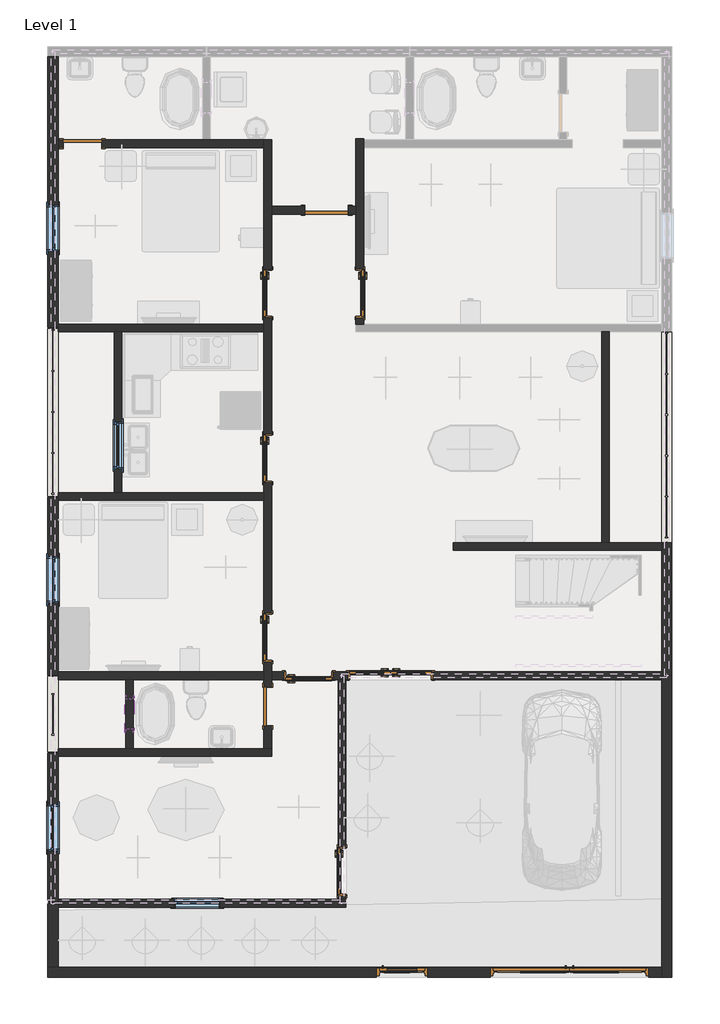
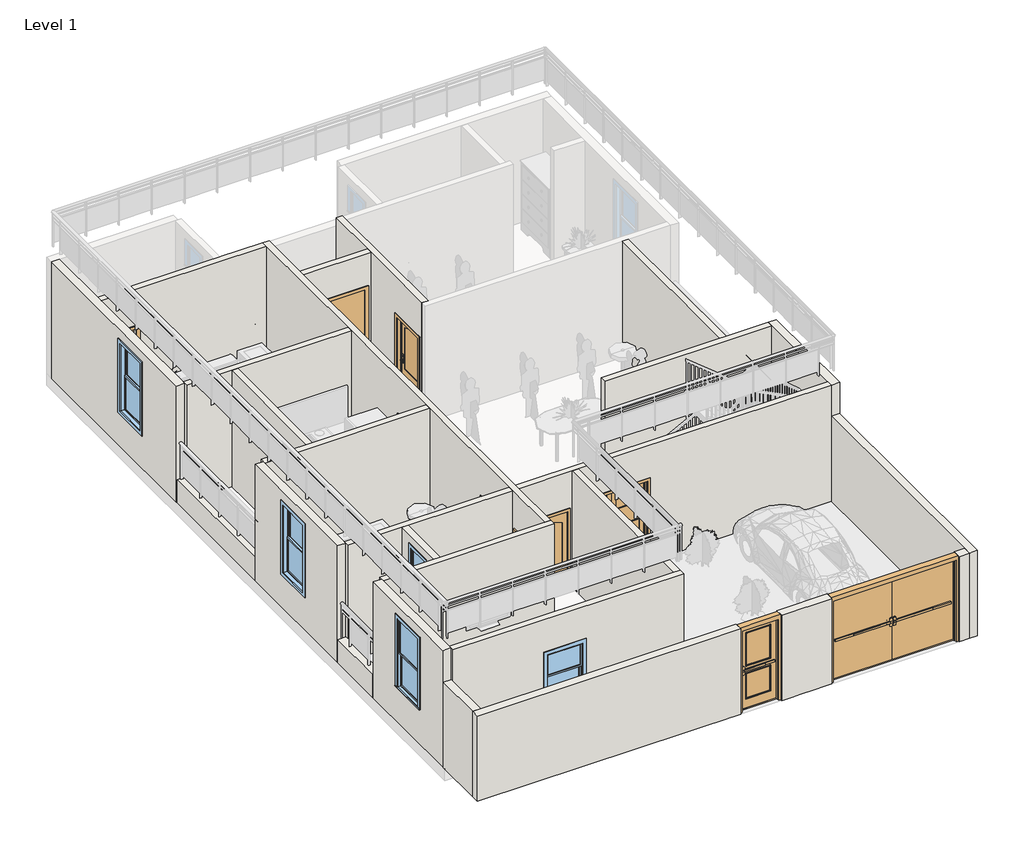
# One storey, part 1 of 6: 25 walls, 12 doors, 6 windows.
"""IFC4 building model written with IfcOpenShell, lengths in millimetres."""

from ifc_helpers import new_model, si_unit, frame, origin, origin_with_axes, place, context, project, spatial, polyline, outline, extrude, faceted_brep, transform, mapped, element, save
from components import door_808aeb8e, door_5d363d20, door_4e55e581, door_5136af5f, door_exterior_single_two_lite_door_exterior_single_two_lite_36a17ea7, door_255cab33, door_059fdd7e, door_99d96fc5, window_d24d93a6, window_d3583dd1, window_3d781103

model = new_model("IFC4")

# Units and contexts
model_context = context("Model", 3, world=origin())
ifc_project = project(units=[si_unit("LENGTHUNIT", "METRE", prefix="MILLI")], contexts=[model_context])

# Site, building, storey
site = spatial("IfcSite", under=ifc_project)
building = spatial("IfcBuilding", under=site)
storey = spatial("IfcBuildingStorey", under=building, Name="Level 1", Elevation=0.0)

# Doors
placement = place(None, origin())
door_shape = door_808aeb8e(model_context)
element("IfcDoor", 1, ObjectType="36\" x 80\"", at=placement, inside=storey, context=model_context, shape_type="MappedRepresentation", body=[
    mapped(door_shape, transform((-10241.5591185, 8951.0271763, 0.0), x_axis=(0.0, 1.0, 0.0), y_axis=(-1.0, 0.0, 0.0), z_axis=(0.0, 0.0, 1.0))),
])
element("IfcDoor", 2, ObjectType="36\" x 80\"", at=placement, inside=storey, context=model_context, shape_type="MappedRepresentation", body=[
    mapped(door_shape, transform((-10241.5591185, 5674.4271763, 0.0), x_axis=(0.0, 1.0, 0.0), y_axis=(-1.0, 0.0, 0.0), z_axis=(0.0, 0.0, 1.0))),
])
element("IfcDoor", 3, ObjectType="36\" x 80\"", at=placement, inside=storey, context=model_context, shape_type="MappedRepresentation", body=[
    mapped(door_shape, transform((-10241.5591185, 2118.4271763, 0.0), x_axis=(0.0, 1.0, 0.0), y_axis=(-1.0, 0.0, 0.0), z_axis=(0.0, 0.0, 1.0))),
])
element("IfcDoor", 4, ObjectType="36\" x 80\"", at=placement, inside=storey, context=model_context, shape_type="MappedRepresentation", body=[
    mapped(door_shape, transform((-9425.5841185, 1353.2521763, 0.0), x_axis=(-1.0, 0.0, 0.0), y_axis=(0.0, -1.0, 0.0), z_axis=(0.0, 0.0, 1.0))),
])
element("IfcDoor", 5, ObjectType="36\" x 80\"", at=placement, inside=storey, context=model_context, shape_type="MappedRepresentation", body=[
    mapped(door_shape, transform((-8768.3591185, -2529.7728237, 0.0), x_axis=(0.0, 1.0, 0.0), y_axis=(-1.0, 0.0, 0.0), z_axis=(0.0, 0.0, 1.0))),
])
door_2_shape = door_5d363d20(model_context)
element("IfcDoor", 6, ObjectType="36\" x 80\"", at=placement, inside=storey, context=model_context, shape_type="MappedRepresentation", body=[
    mapped(door_2_shape, transform((-8406.4091185, 8951.0271763, 0.0), x_axis=(0.0, 1.0, 0.0), y_axis=(-1.0, 0.0, 0.0), z_axis=(0.0, 0.0, 1.0))),
])
door_3_shape = door_4e55e581(model_context)
element("IfcDoor", 7, ObjectType="Door-Exterior-Double : 120\" x 84\"", at=placement, inside=storey, context=model_context, shape_type="MappedRepresentation", body=[
    mapped(door_3_shape, transform((-4243.9841185, -4542.7228237, 0.0), x_axis=(1.0, 0.0, 0.0), y_axis=(0.0, 1.0, 0.0), z_axis=(0.0, 0.0, 1.0))),
])
door_4_shape = door_5136af5f(model_context)
element("IfcDoor", 8, ObjectType="Door-Exterior-Double-Full Glass-Wood_Clad : 64\" x 84\"", at=placement, inside=storey, context=model_context, shape_type="MappedRepresentation", body=[
    mapped(door_4_shape, transform((-7799.9841185, 1359.6021763, 0.0), x_axis=(1.0, 0.0, 0.0), y_axis=(0.0, 1.0, 0.0), z_axis=(0.0, 0.0, 1.0))),
])
door_exterior_single_two_lite_door_exterior_single_two_lite_shape = door_exterior_single_two_lite_door_exterior_single_two_lite_36a17ea7(model_context)
element("IfcDoor", 9, ObjectType="Door-Exterior-Single-Two_Lite : Door-Exterior-Single-Two_Lite", at=placement, inside=storey, context=model_context, shape_type="MappedRepresentation", body=[
    mapped(door_exterior_single_two_lite_door_exterior_single_two_lite_shape, transform((-7571.3841185, -4542.7228237, 0.0), x_axis=(1.0, 0.0, 0.0), y_axis=(0.0, 1.0, 0.0), z_axis=(0.0, 0.0, 1.0))),
])
door_5_shape = door_255cab33(model_context)
element("IfcDoor", 10, ObjectType="Single-Flush : 30\" x 80\"", at=placement, inside=storey, context=model_context, shape_type="MappedRepresentation", body=[
    mapped(door_5_shape, transform((-13921.3841185, 11922.8271763, 0.0), x_axis=(-1.0, 0.0, 0.0), y_axis=(0.0, -1.0, 0.0), z_axis=(0.0, 0.0, 1.0))),
])
door_6_shape = door_059fdd7e(model_context)
element("IfcDoor", 11, ObjectType="Single-Flush : 30\" x 80\"", at=placement, inside=storey, context=model_context, shape_type="MappedRepresentation", body=[
    mapped(door_6_shape, transform((-10238.3841185, 746.8271763, 0.0), x_axis=(0.0, 1.0, 0.0), y_axis=(-1.0, 0.0, 0.0), z_axis=(0.0, 0.0, 1.0))),
])
door_7_shape = door_99d96fc5(model_context)
element("IfcDoor", 12, ObjectType="Single-Flush : 34\" x 84\"", at=placement, inside=storey, context=model_context, shape_type="MappedRepresentation", body=[
    mapped(door_7_shape, transform((-9069.9841185, 10602.0271763, 0.0), x_axis=(1.0, 0.0, 0.0), y_axis=(0.0, 1.0, 0.0), z_axis=(0.0, 0.0, 1.0))),
])

# Walls
element("IfcWall", 13, ObjectType="Generic - 7'2\"", at=placement, inside=storey, context=model_context, shape_type="Brep", body=[
    faceted_brep([(-2415.1841185, -4434.7728237, 2235.2), (-2415.1841185, -4434.7728237, 0.0), (-2669.1841185, -4434.7728237, 0.0), (-2669.1841185, -4434.7728237, 2235.2), (-2415.1841185, -4637.9728237, 0.0), (-2415.1841185, -4637.9728237, 2235.2), (-2669.1841185, -4637.9728237, 2235.2), (-2669.1841185, -4637.9728237, 0.0)], [[[0, 1, 2, 3]], [[4, 5, 6, 7]], [[1, 4, 7, 2]], [[5, 0, 3, 6]], [[1, 0, 5, 4]], [[3, 2, 7, 6]]]),
    faceted_brep([(-14607.1841185, -4434.7728237, 0.0), (-14607.1841185, -4434.7728237, 2235.2), (-14403.9841185, -4434.7728237, 2235.2), (-8079.3841185, -4434.7728237, 2235.2), (-8079.3841185, -4434.7728237, 0.0), (-14403.9841185, -4434.7728237, 0.0), (-14607.1841185, -4637.9728237, 2235.2), (-14607.1841185, -4637.9728237, 0.0), (-8079.3841185, -4637.9728237, 0.0), (-8079.3841185, -4637.9728237, 2235.2)], [[[0, 1, 2, 3, 4, 5]], [[6, 7, 8, 9]], [[7, 0, 5, 4, 8]], [[1, 6, 9, 3, 2]], [[1, 0, 7, 6]], [[4, 3, 9, 8]]]),
    faceted_brep([(-5818.7841185, -4434.7728237, 2235.2), (-5818.7841185, -4434.7728237, 0.0), (-7063.3841185, -4434.7728237, 0.0), (-7063.3841185, -4434.7728237, 2235.2), (-5818.7841185, -4637.9728237, 0.0), (-5818.7841185, -4637.9728237, 2235.2), (-7063.3841185, -4637.9728237, 2235.2), (-7063.3841185, -4637.9728237, 0.0)], [[[0, 1, 2, 3]], [[4, 5, 6, 7]], [[1, 4, 7, 2]], [[5, 0, 3, 6]], [[1, 0, 5, 4]], [[3, 2, 7, 6]]]),
])
element("IfcWall", 14, ObjectType="Generic - 7'2\"", at=placement, inside=storey, context=model_context, shape_type="SweptSolid", body=[
    extrude(outline(polyline([(-14403.9841185, -3177.4728237), (-14403.9841185, -4434.7728237), (-14607.1841185, -4434.7728237), (-14607.1841185, -3177.4728237), (-14403.9841185, -3177.4728237)])), origin_with_axes(), (0.0, 0.0, 1.0), 2235.2),
])
element("IfcWall", 15, ObjectType="Generic - 7'2\"", at=placement, inside=storey, context=model_context, shape_type="Brep", body=[
    faceted_brep([(-2415.1841185, 1356.4271763, 0.0), (-2415.1841185, 1280.2271763, 0.0), (-2415.1841185, -4434.7728237, 0.0), (-2415.1841185, -4637.9728237, 0.0), (-2415.1841185, -4637.9728237, 2235.2), (-2415.1841185, -4434.7728237, 2235.2), (-2415.1841185, 1356.4271763, 2235.2), (-2211.9841185, 1356.4271763, 0.0), (-2211.9841185, 1356.4271763, 2235.2), (-2211.9841185, -4637.9728237, 2235.2), (-2211.9841185, -4637.9728237, 0.0)], [[[0, 1, 2, 3, 4, 5, 6]], [[7, 8, 9, 10]], [[3, 2, 1, 0, 7, 10]], [[6, 5, 4, 9, 8]], [[0, 6, 8, 7]], [[4, 3, 10, 9]]]),
])
element("IfcWall", 16, ObjectType="Generic - 8\"", at=placement, inside=storey, context=model_context, shape_type="Brep", body=[
    faceted_brep([(-14403.9841185, 8277.9271763, 0.0), (-14403.9841185, 8341.4271763, 0.0), (-14403.9841185, 11846.6271763, 0.0), (-14403.9841185, 11999.0271763, 0.0), (-14403.9841185, 13650.0271763, 0.0), (-14403.9841185, 13650.0271763, 3048.0), (-14403.9841185, 11999.0271763, 3048.0), (-14403.9841185, 11846.6271763, 3048.0), (-14403.9841185, 8341.4271763, 3048.0), (-14403.9841185, 8277.9271763, 3048.0), (-14403.9841185, 9789.2271763, 2743.2), (-14403.9841185, 10703.6271763, 2743.2), (-14403.9841185, 10703.6271763, 914.4), (-14403.9841185, 9789.2271763, 914.4), (-14607.1841185, 8277.9271763, 0.0), (-14607.1841185, 8277.9271763, 3048.0), (-14607.1841185, 13650.0271763, 3048.0), (-14607.1841185, 13650.0271763, 0.0), (-14607.1841185, 9789.2271763, 2743.2), (-14607.1841185, 9789.2271763, 914.4), (-14607.1841185, 10703.6271763, 914.4), (-14607.1841185, 10703.6271763, 2743.2)], [[[0, 1, 2, 3, 4, 5, 6, 7, 8, 9], [10, 11, 12, 13]], [[14, 15, 16, 17], [18, 19, 20, 21]], [[4, 3, 2, 1, 0, 14, 17]], [[0, 9, 15, 14]], [[5, 4, 17, 16]], [[18, 21, 11, 10]], [[21, 20, 12, 11]], [[20, 19, 13, 12]], [[19, 18, 10, 13]], [[9, 8, 7, 6, 5, 16, 15]]]),
])
element("IfcWall", 17, ObjectType="Generic - 8\"", at=placement, inside=storey, context=model_context, shape_type="Brep", body=[
    faceted_brep([(-14403.9841185, 4925.1271763, 0.0), (-14403.9841185, 4988.6271763, 0.0), (-14403.9841185, 8252.5271763, 0.0), (-14403.9841185, 8252.5271763, 609.6), (-14403.9841185, 4925.1271763, 609.6), (-14607.1841185, 4925.1271763, 0.0), (-14607.1841185, 4925.1271763, 609.6), (-14607.1841185, 8252.5271763, 609.6), (-14607.1841185, 8252.5271763, 0.0)], [[[0, 1, 2, 3, 4]], [[5, 6, 7, 8]], [[2, 1, 0, 5, 8]], [[3, 2, 8, 7]], [[4, 3, 7, 6]], [[0, 4, 6, 5]]]),
])
element("IfcWall", 18, ObjectType="Generic - 8\"", at=placement, inside=storey, context=model_context, shape_type="Brep", body=[
    faceted_brep([(-14403.9841185, 1369.1271763, 0.0), (-14403.9841185, 1432.6271763, 0.0), (-14403.9841185, 4899.7271763, 0.0), (-14403.9841185, 4899.7271763, 3048.0), (-14403.9841185, 1432.6271763, 3048.0), (-14403.9841185, 1369.1271763, 3048.0), (-14403.9841185, 2804.2271763, 2743.2), (-14403.9841185, 3718.6271763, 2743.2), (-14403.9841185, 3718.6271763, 914.4), (-14403.9841185, 2804.2271763, 914.4), (-14607.1841185, 1369.1271763, 0.0), (-14607.1841185, 1369.1271763, 3048.0), (-14607.1841185, 4899.7271763, 3048.0), (-14607.1841185, 4899.7271763, 0.0), (-14607.1841185, 2804.2271763, 2743.2), (-14607.1841185, 2804.2271763, 914.4), (-14607.1841185, 3718.6271763, 914.4), (-14607.1841185, 3718.6271763, 2743.2)], [[[0, 1, 2, 3, 4, 5], [6, 7, 8, 9]], [[10, 11, 12, 13], [14, 15, 16, 17]], [[2, 1, 0, 10, 13]], [[3, 2, 13, 12]], [[0, 5, 11, 10]], [[14, 17, 7, 6]], [[17, 16, 8, 7]], [[16, 15, 9, 8]], [[15, 14, 6, 9]], [[5, 4, 3, 12, 11]]]),
])
element("IfcWall", 19, ObjectType="Generic - 8\"", at=placement, inside=storey, context=model_context, shape_type="Brep", body=[
    faceted_brep([(-14403.9841185, -154.8728237, 0.0), (-14403.9841185, -91.3728237, 0.0), (-14403.9841185, 1343.7271763, 0.0), (-14403.9841185, 1343.7271763, 609.6), (-14403.9841185, -154.8728237, 609.6), (-14607.1841185, -154.8728237, 0.0), (-14607.1841185, -154.8728237, 609.6), (-14607.1841185, 1343.7271763, 609.6), (-14607.1841185, 1343.7271763, 0.0)], [[[0, 1, 2, 3, 4]], [[5, 6, 7, 8]], [[2, 1, 0, 5, 8]], [[3, 2, 8, 7]], [[4, 3, 7, 6]], [[0, 4, 6, 5]]]),
])
element("IfcWall", 20, ObjectType="Generic - 8\"", at=placement, inside=storey, context=model_context, shape_type="Brep", body=[
    faceted_brep([(-2415.1841185, 8265.2271763, 0.0), (-2415.1841185, 8189.0271763, 0.0), (-2415.1841185, 3998.0271763, 0.0), (-2415.1841185, 3921.8271763, 0.0), (-2415.1841185, 3921.8271763, 609.6), (-2415.1841185, 3998.0271763, 609.6), (-2415.1841185, 8189.0271763, 609.6), (-2415.1841185, 8265.2271763, 609.6), (-2211.9841185, 8265.2271763, 0.0), (-2211.9841185, 8265.2271763, 609.6), (-2211.9841185, 8189.0271763, 609.6), (-2211.9841185, 3998.0271763, 609.6), (-2211.9841185, 3921.8271763, 609.6), (-2211.9841185, 3921.8271763, 0.0)], [[[0, 1, 2, 3, 4, 5, 6, 7]], [[8, 9, 10, 11, 12, 13]], [[3, 2, 1, 0, 8, 13]], [[4, 3, 13, 12]], [[7, 6, 5, 4, 12, 11, 10, 9]], [[0, 7, 9, 8]]]),
])
element("IfcWall", 21, ObjectType="Generic - 8\"", at=placement, inside=storey, context=model_context, shape_type="Brep", body=[
    faceted_brep([(-2415.1841185, 3921.8271763, 0.0), (-2415.1841185, 3845.6271763, 0.0), (-2415.1841185, 1432.6271763, 0.0), (-2415.1841185, 1356.4271763, 0.0), (-2415.1841185, 1356.4271763, 2235.2), (-2415.1841185, 1280.2271763, 2235.2), (-2415.1841185, 1280.2271763, 3048.0), (-2415.1841185, 1432.6271763, 3048.0), (-2415.1841185, 3845.6271763, 3048.0), (-2415.1841185, 3998.0271763, 3048.0), (-2415.1841185, 3998.0271763, 609.6), (-2415.1841185, 3921.8271763, 609.6), (-2211.9841185, 3921.8271763, 0.0), (-2211.9841185, 3921.8271763, 609.6), (-2211.9841185, 3998.0271763, 609.6), (-2211.9841185, 3998.0271763, 3048.0), (-2211.9841185, 1280.2271763, 3048.0), (-2211.9841185, 1280.2271763, 2235.2), (-2211.9841185, 1356.4271763, 2235.2), (-2211.9841185, 1356.4271763, 0.0)], [[[0, 1, 2, 3, 4, 5, 6, 7, 8, 9, 10, 11]], [[12, 13, 14, 15, 16, 17, 18, 19]], [[3, 2, 1, 0, 12, 19]], [[0, 11, 13, 12]], [[10, 14, 13, 11]], [[10, 9, 15, 14]], [[4, 3, 19, 18]], [[17, 5, 4, 18]], [[6, 5, 17, 16]], [[9, 8, 7, 6, 16, 15]]]),
])
element("IfcWall", 22, ObjectType="Generic - 8\"", at=placement, inside=storey, context=model_context, shape_type="Brep", body=[
    faceted_brep([(-14403.9841185, -3152.0728237, 0.0), (-14403.9841185, -3088.5728237, 0.0), (-14403.9841185, -180.2728237, 0.0), (-14403.9841185, -180.2728237, 3048.0), (-14403.9841185, -3088.5728237, 3048.0), (-14403.9841185, -3152.0728237, 3048.0), (-14403.9841185, -1208.9728237, 2743.2), (-14403.9841185, -1208.9728237, 914.4), (-14403.9841185, -2123.3728237, 914.4), (-14403.9841185, -2123.3728237, 2743.2), (-14607.1841185, -3152.0728237, 0.0), (-14607.1841185, -3152.0728237, 3048.0), (-14607.1841185, -180.2728237, 3048.0), (-14607.1841185, -180.2728237, 0.0), (-14607.1841185, -1208.9728237, 2743.2), (-14607.1841185, -2123.3728237, 2743.2), (-14607.1841185, -2123.3728237, 914.4), (-14607.1841185, -1208.9728237, 914.4)], [[[0, 1, 2, 3, 4, 5], [6, 7, 8, 9]], [[10, 11, 12, 13], [14, 15, 16, 17]], [[2, 1, 0, 10, 13]], [[3, 2, 13, 12]], [[0, 5, 11, 10]], [[6, 9, 15, 14]], [[9, 8, 16, 15]], [[8, 7, 17, 16]], [[7, 6, 14, 17]], [[5, 4, 3, 12, 11]]]),
])
element("IfcWall", 23, ObjectType="INNER -6\"", at=placement, inside=storey, context=model_context, shape_type="Brep", body=[
    faceted_brep([(-14403.9841185, 11846.6271763, 0.0), (-14302.3841185, 11846.6271763, 0.0), (-14302.3841185, 11846.6271763, 2032.0), (-13540.3841185, 11846.6271763, 2032.0), (-13540.3841185, 11846.6271763, 0.0), (-10314.5841185, 11846.6271763, 0.0), (-10314.5841185, 11846.6271763, 3048.0), (-14403.9841185, 11846.6271763, 3048.0), (-14302.3841185, 11999.0271763, 2032.0), (-14302.3841185, 11999.0271763, 0.0), (-14403.9841185, 11999.0271763, 0.0), (-14403.9841185, 11999.0271763, 3048.0), (-11533.7841185, 11999.0271763, 3048.0), (-11381.3841185, 11999.0271763, 3048.0), (-10314.5841185, 11999.0271763, 3048.0), (-10314.5841185, 11999.0271763, 0.0), (-11381.3841185, 11999.0271763, 0.0), (-11533.7841185, 11999.0271763, 0.0), (-13540.3841185, 11999.0271763, 0.0), (-13540.3841185, 11999.0271763, 2032.0)], [[[0, 1, 2, 3, 4, 5, 6, 7]], [[8, 9, 10, 11, 12, 13, 14, 15, 16, 17, 18, 19]], [[10, 9, 1, 0]], [[18, 17, 16, 15, 5, 4]], [[0, 7, 11, 10]], [[6, 5, 15, 14]], [[2, 1, 9, 8]], [[3, 2, 8, 19]], [[4, 3, 19, 18]], [[7, 6, 14, 13, 12, 11]]]),
])
element("IfcWall", 24, ObjectType="INNER -6\"", at=placement, inside=storey, context=model_context, shape_type="Brep", body=[
    faceted_brep([(-14403.9841185, 8189.0271763, 0.0), (-13286.3841185, 8189.0271763, 0.0), (-13133.9841185, 8189.0271763, 0.0), (-10314.5841185, 8189.0271763, 0.0), (-10314.5841185, 8189.0271763, 3048.0), (-13133.9841185, 8189.0271763, 3048.0), (-13286.3841185, 8189.0271763, 3048.0), (-14403.9841185, 8189.0271763, 3048.0), (-14403.9841185, 8341.4271763, 0.0), (-14403.9841185, 8341.4271763, 3048.0), (-10314.5841185, 8341.4271763, 3048.0), (-10314.5841185, 8341.4271763, 0.0), (-14403.9841185, 8277.9271763, 0.0), (-14403.9841185, 8277.9271763, 3048.0)], [[[0, 1, 2, 3, 4, 5, 6, 7]], [[8, 9, 10, 11]], [[3, 2, 1, 0, 12, 8, 11]], [[0, 7, 13, 9, 8, 12]], [[4, 3, 11, 10]], [[7, 6, 5, 4, 10, 9, 13]]]),
])
element("IfcWall", 25, ObjectType="INNER -6\"", at=placement, inside=storey, context=model_context, shape_type="Brep", body=[
    faceted_brep([(-10162.1841185, 1127.8271763, 2032.0), (-10162.1841185, 1127.8271763, 0.0), (-10162.1841185, 1280.2271763, 0.0), (-10162.1841185, 1432.6271763, 0.0), (-10162.1841185, 1635.8271763, 0.0), (-10162.1841185, 1635.8271763, 2057.4), (-10162.1841185, 2601.0271763, 2057.4), (-10162.1841185, 2601.0271763, 0.0), (-10162.1841185, 5191.8271763, 0.0), (-10162.1841185, 5191.8271763, 2057.4), (-10162.1841185, 6157.0271763, 2057.4), (-10162.1841185, 6157.0271763, 0.0), (-10162.1841185, 8468.4271763, 0.0), (-10162.1841185, 8468.4271763, 2057.4), (-10162.1841185, 9433.6271763, 2057.4), (-10162.1841185, 9433.6271763, 0.0), (-10162.1841185, 10525.8271763, 0.0), (-10162.1841185, 10678.2271763, 0.0), (-10162.1841185, 11999.0271763, 0.0), (-10162.1841185, 11999.0271763, 3048.0), (-10162.1841185, 10678.2271763, 3048.0), (-10162.1841185, 10525.8271763, 3048.0), (-10162.1841185, 1432.6271763, 3048.0), (-10162.1841185, 1280.2271763, 3048.0), (-10162.1841185, -91.3728237, 3048.0), (-10162.1841185, -91.3728237, 0.0), (-10162.1841185, 365.8271763, 0.0), (-10162.1841185, 365.8271763, 2032.0), (-10314.5841185, 1635.8271763, 0.0), (-10314.5841185, 1432.6271763, 0.0), (-10314.5841185, 1280.2271763, 0.0), (-10314.5841185, 1127.8271763, 0.0), (-10314.5841185, 1127.8271763, 2032.0), (-10314.5841185, 365.8271763, 2032.0), (-10314.5841185, 365.8271763, 0.0), (-10314.5841185, -91.3728237, 0.0), (-10314.5841185, -91.3728237, 3048.0), (-10314.5841185, 1280.2271763, 3048.0), (-10314.5841185, 1432.6271763, 3048.0), (-10314.5841185, 4836.2271763, 3048.0), (-10314.5841185, 4988.6271763, 3048.0), (-10314.5841185, 8189.0271763, 3048.0), (-10314.5841185, 8341.4271763, 3048.0), (-10314.5841185, 11846.6271763, 3048.0), (-10314.5841185, 11999.0271763, 3048.0), (-10314.5841185, 11999.0271763, 0.0), (-10314.5841185, 11846.6271763, 0.0), (-10314.5841185, 9433.6271763, 0.0), (-10314.5841185, 9433.6271763, 2057.4), (-10314.5841185, 8468.4271763, 2057.4), (-10314.5841185, 8468.4271763, 0.0), (-10314.5841185, 8341.4271763, 0.0), (-10314.5841185, 8189.0271763, 0.0), (-10314.5841185, 6157.0271763, 0.0), (-10314.5841185, 6157.0271763, 2057.4), (-10314.5841185, 5191.8271763, 2057.4), (-10314.5841185, 5191.8271763, 0.0), (-10314.5841185, 4988.6271763, 0.0), (-10314.5841185, 4836.2271763, 0.0), (-10314.5841185, 2601.0271763, 0.0), (-10314.5841185, 2601.0271763, 2057.4), (-10314.5841185, 1635.8271763, 2057.4)], [[[0, 1, 2, 3, 4, 5, 6, 7, 8, 9, 10, 11, 12, 13, 14, 15, 16, 17, 18, 19, 20, 21, 22, 23, 24, 25, 26, 27]], [[28, 29, 30, 31, 32, 33, 34, 35, 36, 37, 38, 39, 40, 41, 42, 43, 44, 45, 46, 47, 48, 49, 50, 51, 52, 53, 54, 55, 56, 57, 58, 59, 60, 61]], [[45, 18, 17, 16, 15, 47, 46]], [[50, 12, 11, 53, 52, 51]], [[56, 8, 7, 59, 58, 57]], [[26, 25, 35, 34]], [[4, 3, 2, 1, 31, 30, 29, 28]], [[19, 18, 45, 44]], [[25, 24, 36, 35]], [[14, 48, 47, 15]], [[48, 14, 13, 49]], [[49, 13, 12, 50]], [[10, 54, 53, 11]], [[54, 10, 9, 55]], [[55, 9, 8, 56]], [[6, 60, 59, 7]], [[60, 6, 5, 61]], [[61, 5, 4, 28]], [[32, 31, 1, 0]], [[33, 32, 0, 27]], [[34, 33, 27, 26]], [[24, 23, 22, 21, 20, 19, 44, 43, 42, 41, 40, 39, 38, 37, 36]]]),
])
element("IfcWall", 26, ObjectType="INNER -6\"", at=placement, inside=storey, context=model_context, shape_type="Brep", body=[
    faceted_brep([(-8485.7841185, 12024.4271763, 3048.0), (-8485.7841185, 12024.4271763, 0.0), (-8485.7841185, 10678.2271763, 0.0), (-8485.7841185, 10525.8271763, 0.0), (-8485.7841185, 9433.6271763, 0.0), (-8485.7841185, 9433.6271763, 2057.4), (-8485.7841185, 8468.4271763, 2057.4), (-8485.7841185, 8468.4271763, 0.0), (-8485.7841185, 8341.4271763, 0.0), (-8485.7841185, 8341.4271763, 3048.0), (-8485.7841185, 10525.8271763, 3048.0), (-8485.7841185, 10678.2271763, 3048.0), (-8333.3841185, 12024.4271763, 0.0), (-8333.3841185, 12024.4271763, 3048.0), (-8333.3841185, 11999.0271763, 3048.0), (-8333.3841185, 11846.6271763, 3048.0), (-8333.3841185, 8341.4271763, 3048.0), (-8333.3841185, 8341.4271763, 0.0), (-8333.3841185, 8468.4271763, 0.0), (-8333.3841185, 8468.4271763, 2057.4), (-8333.3841185, 9433.6271763, 2057.4), (-8333.3841185, 9433.6271763, 0.0), (-8333.3841185, 11846.6271763, 0.0), (-8333.3841185, 11999.0271763, 0.0)], [[[0, 1, 2, 3, 4, 5, 6, 7, 8, 9, 10, 11]], [[12, 13, 14, 15, 16, 17, 18, 19, 20, 21, 22, 23]], [[1, 12, 23, 22, 21, 4, 3, 2]], [[17, 8, 7, 18]], [[1, 0, 13, 12]], [[9, 8, 17, 16]], [[20, 5, 4, 21]], [[5, 20, 19, 6]], [[6, 19, 18, 7]], [[0, 11, 10, 9, 16, 15, 14, 13]]]),
])
element("IfcWall", 27, ObjectType="INNER -6\"", at=placement, inside=storey, context=model_context, shape_type="Brep", body=[
    faceted_brep([(-10314.5841185, 4988.6271763, 0.0), (-13133.9841185, 4988.6271763, 0.0), (-13286.3841185, 4988.6271763, 0.0), (-14403.9841185, 4988.6271763, 0.0), (-14403.9841185, 4988.6271763, 3048.0), (-13286.3841185, 4988.6271763, 3048.0), (-13133.9841185, 4988.6271763, 3048.0), (-10314.5841185, 4988.6271763, 3048.0), (-10314.5841185, 4836.2271763, 0.0), (-10314.5841185, 4836.2271763, 3048.0), (-14403.9841185, 4836.2271763, 3048.0), (-14403.9841185, 4836.2271763, 0.0), (-14403.9841185, 4925.1271763, 0.0)], [[[0, 1, 2, 3, 4, 5, 6, 7]], [[8, 9, 10, 11]], [[3, 2, 1, 0, 8, 11, 12]], [[0, 7, 9, 8]], [[4, 3, 12, 11, 10]], [[7, 6, 5, 4, 10, 9]]]),
])
element("IfcWall", 28, ObjectType="INNER -6\"", at=placement, inside=storey, context=model_context, shape_type="SweptSolid", body=[
    extrude(outline(polyline([(4988.6271763, 0.0), (4988.6271763, 3048.0), (8189.0271763, 3048.0), (8189.0271763, 0.0), (4988.6271763, 0.0)]), holes=[polyline([(5471.2271763, 2184.4), (5471.2271763, 965.2), (6385.6271763, 965.2), (6385.6271763, 2184.4), (5471.2271763, 2184.4)])]), frame((-13286.3841185, 0.0, 0.0), z_axis=(1.0, 0.0, 0.0), x_axis=(0.0, 1.0, 0.0)), (0.0, 0.0, 1.0), 152.4),
])
element("IfcWall", 29, ObjectType="INNER -6\"", at=placement, inside=storey, context=model_context, shape_type="Brep", body=[
    faceted_brep([(-10314.5841185, 1432.6271763, 0.0), (-14403.9841185, 1432.6271763, 0.0), (-14403.9841185, 1432.6271763, 3048.0), (-10314.5841185, 1432.6271763, 3048.0), (-10314.5841185, 1280.2271763, 0.0), (-10314.5841185, 1280.2271763, 3048.0), (-12905.3841185, 1280.2271763, 3048.0), (-13057.7841185, 1280.2271763, 3048.0), (-14403.9841185, 1280.2271763, 3048.0), (-14403.9841185, 1280.2271763, 0.0), (-13057.7841185, 1280.2271763, 0.0), (-12905.3841185, 1280.2271763, 0.0), (-14403.9841185, 1369.1271763, 0.0), (-14403.9841185, 1369.1271763, 3048.0)], [[[0, 1, 2, 3]], [[4, 5, 6, 7, 8, 9, 10, 11]], [[1, 0, 4, 11, 10, 9, 12]], [[0, 3, 5, 4]], [[2, 1, 12, 9, 8, 13]], [[3, 2, 13, 8, 7, 6, 5]]]),
])
element("IfcWall", 30, ObjectType="INNER -6\"", at=placement, inside=storey, context=model_context, shape_type="SweptSolid", body=[
    extrude(outline(polyline([(-91.3728237, 0.0), (-91.3728237, 3048.0), (1280.2271763, 3048.0), (1280.2271763, 0.0), (-91.3728237, 0.0)]), holes=[polyline([(899.2271763, 2768.6), (289.6271763, 2768.6), (289.6271763, 2159.0), (899.2271763, 2159.0), (899.2271763, 2768.6)])]), frame((-13057.7841185, 0.0, 0.0), z_axis=(1.0, 0.0, 0.0), x_axis=(0.0, 1.0, 0.0)), (0.0, 0.0, 1.0), 152.4),
])
element("IfcWall", 31, ObjectType="INNER -6\"", at=placement, inside=storey, context=model_context, shape_type="Brep", body=[
    faceted_brep([(-14403.9841185, -3240.9728237, 0.0), (-8688.9841185, -3240.9728237, 0.0), (-8688.9841185, -3240.9728237, 3048.0), (-14403.9841185, -3240.9728237, 3048.0), (-12092.5841185, -3240.9728237, 2133.6), (-11178.1841185, -3240.9728237, 2133.6), (-11178.1841185, -3240.9728237, 914.4), (-12092.5841185, -3240.9728237, 914.4), (-14403.9841185, -3088.5728237, 0.0), (-14403.9841185, -3088.5728237, 3048.0), (-8841.3841185, -3088.5728237, 3048.0), (-8688.9841185, -3088.5728237, 3048.0), (-8688.9841185, -3088.5728237, 0.0), (-8841.3841185, -3088.5728237, 0.0), (-12092.5841185, -3088.5728237, 2133.6), (-12092.5841185, -3088.5728237, 914.4), (-11178.1841185, -3088.5728237, 914.4), (-11178.1841185, -3088.5728237, 2133.6), (-14403.9841185, -3152.0728237, 0.0), (-14403.9841185, -3152.0728237, 3048.0)], [[[0, 1, 2, 3], [4, 5, 6, 7]], [[8, 9, 10, 11, 12, 13], [14, 15, 16, 17]], [[1, 0, 18, 8, 13, 12]], [[0, 3, 19, 9, 8, 18]], [[2, 1, 12, 11]], [[15, 14, 4, 7]], [[16, 15, 7, 6]], [[17, 16, 6, 5]], [[14, 17, 5, 4]], [[3, 2, 11, 10, 9, 19]]]),
])
element("IfcWall", 32, ObjectType="INNER -6\"", at=placement, inside=storey, context=model_context, shape_type="SweptSolid", body=[
    extrude(outline(polyline([(-3088.5728237, 0.0), (-3088.5728237, 3048.0), (1280.2271763, 3048.0), (1280.2271763, 0.0), (-2047.1728237, 0.0), (-2047.1728237, 2057.4), (-3012.3728237, 2057.4), (-3012.3728237, 0.0), (-3088.5728237, 0.0)])), frame((-8841.3841185, 0.0, 0.0), z_axis=(1.0, 0.0, 0.0), x_axis=(0.0, 1.0, 0.0)), (0.0, 0.0, 1.0), 152.4),
])
element("IfcWall", 33, ObjectType="INNER -6\"", at=placement, inside=storey, context=model_context, shape_type="Brep", body=[
    faceted_brep([(-2415.1841185, 3998.0271763, 3048.0), (-2415.1841185, 3998.0271763, 609.6), (-2415.1841185, 3998.0271763, 0.0), (-3456.5841185, 3998.0271763, 0.0), (-3608.9841185, 3998.0271763, 0.0), (-6555.3841185, 3998.0271763, 0.0), (-6555.3841185, 3998.0271763, 3048.0), (-3608.9841185, 3998.0271763, 3048.0), (-3456.5841185, 3998.0271763, 3048.0), (-2415.1841185, 3845.6271763, 0.0), (-2415.1841185, 3845.6271763, 3048.0), (-6555.3841185, 3845.6271763, 3048.0), (-6555.3841185, 3845.6271763, 0.0), (-2415.1841185, 3921.8271763, 0.0)], [[[0, 1, 2, 3, 4, 5, 6, 7, 8]], [[9, 10, 11, 12]], [[5, 4, 3, 2, 13, 9, 12]], [[6, 5, 12, 11]], [[0, 10, 9, 13, 2, 1]], [[0, 8, 7, 6, 11, 10]]]),
])
element("IfcWall", 34, ObjectType="INNER -6\"", at=placement, inside=storey, context=model_context, shape_type="SweptSolid", body=[
    extrude(outline(polyline([(-3608.9841185, 3998.0271763), (-3608.9841185, 8189.0271763), (-3456.5841185, 8189.0271763), (-3456.5841185, 3998.0271763), (-3608.9841185, 3998.0271763)])), origin_with_axes(), (0.0, 0.0, 1.0), 3048.0),
])
element("IfcWall", 35, ObjectType="INNER -6\"", at=placement, inside=storey, context=model_context, shape_type="SweptSolid", body=[
    extrude(outline(polyline([(2133.6, -8638.1841185), (0.0, -8638.1841185), (0.0, -8485.7841185), (3048.0, -8485.7841185), (3048.0, -10162.1841185), (0.0, -10162.1841185), (0.0, -9501.7841185), (2133.6, -9501.7841185), (2133.6, -8638.1841185)])), frame((0.0, 10525.8271763, 0.0), z_axis=(0.0, 1.0, 0.0), x_axis=(0.0, 0.0, 1.0)), (0.0, 0.0, 1.0), 152.4),
])
element("IfcWall", 36, ObjectType="INNER -6\"", at=placement, inside=storey, context=model_context, shape_type="Brep", body=[
    faceted_brep([(-10162.1841185, -91.3728237, 0.0), (-10314.5841185, -91.3728237, 0.0), (-12905.3841185, -91.3728237, 0.0), (-13057.7841185, -91.3728237, 0.0), (-14403.9841185, -91.3728237, 0.0), (-14403.9841185, -91.3728237, 3048.0), (-13057.7841185, -91.3728237, 3048.0), (-12905.3841185, -91.3728237, 3048.0), (-10314.5841185, -91.3728237, 3048.0), (-10162.1841185, -91.3728237, 3048.0), (-10162.1841185, -243.7728237, 0.0), (-10162.1841185, -243.7728237, 3048.0), (-14403.9841185, -243.7728237, 3048.0), (-14403.9841185, -243.7728237, 0.0), (-14403.9841185, -154.8728237, 0.0)], [[[0, 1, 2, 3, 4, 5, 6, 7, 8, 9]], [[10, 11, 12, 13]], [[4, 3, 2, 1, 0, 10, 13, 14]], [[5, 4, 14, 13, 12]], [[0, 9, 11, 10]], [[9, 8, 7, 6, 5, 12, 11]]]),
])
element("IfcWall", 37, ObjectType="INNER -6\"", at=placement, inside=storey, context=model_context, shape_type="Brep", body=[
    faceted_brep([(-10162.1841185, 1280.2271763, 3048.0), (-10162.1841185, 1280.2271763, 0.0), (-9908.1841185, 1280.2271763, 0.0), (-9908.1841185, 1280.2271763, 2057.4), (-8942.9841185, 1280.2271763, 2057.4), (-8942.9841185, 1280.2271763, 0.0), (-8841.3841185, 1280.2271763, 0.0), (-8688.9841185, 1280.2271763, 0.0), (-8638.1841185, 1280.2271763, 0.0), (-8638.1841185, 1280.2271763, 2159.0), (-6961.7841185, 1280.2271763, 2159.0), (-6961.7841185, 1280.2271763, 0.0), (-2415.1841185, 1280.2271763, 0.0), (-2415.1841185, 1280.2271763, 2235.2), (-2415.1841185, 1280.2271763, 3048.0), (-8682.6341185, 1280.2271763, 3048.0), (-8688.9841185, 1280.2271763, 3048.0), (-8841.3841185, 1280.2271763, 3048.0), (-10162.1841185, 1432.6271763, 3048.0), (-2415.1841185, 1432.6271763, 3048.0), (-2415.1841185, 1432.6271763, 0.0), (-6961.7841185, 1432.6271763, 0.0), (-6961.7841185, 1432.6271763, 2159.0), (-8638.1841185, 1432.6271763, 2159.0), (-8638.1841185, 1432.6271763, 0.0), (-8942.9841185, 1432.6271763, 0.0), (-8942.9841185, 1432.6271763, 2057.4), (-9908.1841185, 1432.6271763, 2057.4), (-9908.1841185, 1432.6271763, 0.0), (-10162.1841185, 1432.6271763, 0.0), (-2415.1841185, 1356.4271763, 0.0)], [[[0, 1, 2, 3, 4, 5, 6, 7, 8, 9, 10, 11, 12, 13, 14, 15, 16, 17]], [[18, 19, 20, 21, 22, 23, 24, 25, 26, 27, 28, 29]], [[1, 29, 28, 2]], [[5, 25, 24, 8, 7, 6]], [[20, 30, 12, 11, 21]], [[1, 0, 18, 29]], [[27, 3, 2, 28]], [[3, 27, 26, 4]], [[4, 26, 25, 5]], [[10, 22, 21, 11]], [[22, 10, 9, 23]], [[23, 9, 8, 24]], [[12, 30, 20, 19, 14, 13]], [[19, 18, 0, 17, 16, 15, 14]]]),
])

# Windows
window_shape = window_d24d93a6(model_context)
element("IfcWindow", 38, ObjectType="Double Hung with Trim : 36\" x 48\"", at=placement, inside=storey, context=model_context, shape_type="MappedRepresentation", body=[
    mapped(window_shape, transform((-11635.3841185, -3164.7728237, 0.0), x_axis=(-1.0, 0.0, 0.0), y_axis=(0.0, -1.0, 0.0), z_axis=(0.0, 0.0, 1.0))),
])
element("IfcWindow", 39, ObjectType="Double Hung with Trim : 36\" x 48\"", at=placement, inside=storey, context=model_context, shape_type="MappedRepresentation", body=[
    mapped(window_shape, transform((-13210.1841185, 5928.4271763, 50.8), x_axis=(0.0, -1.0, 0.0), y_axis=(1.0, 0.0, 0.0), z_axis=(0.0, 0.0, 1.0))),
])
window_2_shape = window_d3583dd1(model_context)
element("IfcWindow", 40, ObjectType="Double Hung with Trim : 36\" x 72\"", at=placement, inside=storey, context=model_context, shape_type="MappedRepresentation", body=[
    mapped(window_2_shape, transform((-14505.5841185, 10246.4271763, 609.6), x_axis=(0.0, -1.0, 0.0), y_axis=(1.0, 0.0, 0.0), z_axis=(0.0, 0.0, 1.0))),
])
element("IfcWindow", 41, ObjectType="Double Hung with Trim : 36\" x 72\"", at=placement, inside=storey, context=model_context, shape_type="MappedRepresentation", body=[
    mapped(window_2_shape, transform((-14505.5841185, -1666.1728237, 609.6), x_axis=(0.0, 1.0, 0.0), y_axis=(-1.0, 0.0, 0.0), z_axis=(0.0, 0.0, 1.0))),
])
element("IfcWindow", 42, ObjectType="Double Hung with Trim : 36\" x 72\"", at=placement, inside=storey, context=model_context, shape_type="MappedRepresentation", body=[
    mapped(window_2_shape, transform((-14505.5841185, 3261.4271763, 609.6), x_axis=(0.0, -1.0, 0.0), y_axis=(1.0, 0.0, 0.0), z_axis=(0.0, 0.0, 1.0))),
])
window_3_shape = window_3d781103(model_context)
element("IfcWindow", 43, ObjectType="Transom with Trim : 24\" x 24\"", at=placement, inside=storey, context=model_context, shape_type="MappedRepresentation", body=[
    mapped(window_3_shape, transform((-12981.5841185, 632.5271763, 0.0), x_axis=(0.0, 1.0, 0.0), y_axis=(-1.0, 0.0, 0.0), z_axis=(0.0, 0.0, 1.0))),
])

save(model, "model.ifc")

# Revit data of these elements
# Type "36\" x 80\""
#   Type Mark = "8"
#   Assembly Code = "B2030100"
#   Analytic Construction = "French door, wood frame with single glass"
#   Threshold Offset [instance default] = 0' - 0 1/2"
#   Thickness = 0' - 1 3/8"
#   Thermal Resistance (R) = 1.0696 (h·ft²·°F)/BTU
#   Swing Angle [instance default] = 90.00°
#   Stiles = 0' - 4 3/4"
#   Rough Width = 3' - 2"
#   Rough Height = 6' - 9"
#   Radius = 1' - 8.05625"
#   Lock Rail = 0' - 7 1/8"
#   Height = 6' - 8"
#   Width = 3' - 0"
#   Heat Transfer Coefficient (U) = 0.9350 BTU/(h·ft²·°F)
#   Door Offset [instance default] = 0' - 0"
#   Bottom Rail = 0' - 9 1/2"
#   Threshold [instance default] = yes
#   Function = 1
#   Exterior Trim [instance default] = yes
#   Trim Material = Cherry
#   Threshold Material = Cherry
#   Panel Material = Cherry
#   Glazing = Glass
#   Frame Material = Cherry
#   Door Handle Material = Aluminum
#   Visual Light Transmittance = 0
#   Solar Heat Gain Coefficient = 0
#   Wall Closure = (empty or 0)
#   Construction Type = (empty or 0)
# Type "Door-Exterior-Double : 120\" x 84\""
#   Type Mark = "11"
#   Assembly Code = "B2030200"
#   Analytic Construction = "Metal"
#   Threshold Length [instance default] = 10' - 4"
#   Threshold Offset [instance default] = 0' - 0 1/2"
#   Thickness = 0' - 1 3/4"
#   Thermal Resistance (R) = 1.5338 (h·ft²·°F)/BTU
#   Swing Angle [instance default] = 90.00°
#   Strike Height = 3' - 4"
#   SinglePanelWidth = 5' - 0"
#   Rough Width [instance default] = 10' - 4"
#   Rough Height [instance default] = 7' - 4"
#   MFOpeningHeight [instance default] = 0' - 4"
#   MFOpeningWidth [instance default] = 0' - 4"
#   Inset Calculate [instance default] = 0' - 4"
#   Masonry Inset [instance default] = 0' - 1"
#   Height = 7' - 0"
#   Width = 10' - 0"
#   Heat Transfer Coefficient (U) = 0.6520 BTU/(h·ft²·°F)
#   Masonry Frame Depth = 0' - 5 3/4"
#   Threshold [instance default] = yes
#   Masonry Frame [instance default] = yes
#   Function = 1
#   Dry Wall Frame [instance default] = no
#   Threshold Material = Cherry
#   Panic Bar Material = Metal - Stainless Steel
#   Panel Material = Metal Door - Brindle
#   Frame Material = Metal - Painted - Grey
#   Exterior Pull Material = Metal - Stainless Steel
#   Visual Light Transmittance = 0
#   Solar Heat Gain Coefficient = 0
#   Wall Closure = (empty or 0)
# Type "Door-Exterior-Double-Full Glass-Wood_Clad : 64\" x 84\""
#   Type Mark = "9"
#   Assembly Code = "B2030100"
#   Analytic Construction = "French door, wood frame with double glass"
#   Top Rail = 0' - 4 11/16"
#   Threshold Offset [instance default] = 0' - 0 1/2"
#   Thickness = 0' - 1 3/8"
#   Thermal Resistance (R) = 1.9158 (h·ft²·°F)/BTU
#   Swing Angle [instance default] = 90.00°
#   Stiles = 0' - 4 3/4"
#   Rough Width = 5' - 6"
#   Rough Height = 7' - 1"
#   Panel Width = 2' - 8"
#   Door Offset [instance default] = 0' - 0"
#   Height = 7' - 0"
#   Width = 5' - 4"
#   Heat Transfer Coefficient (U) = 0.5220 BTU/(h·ft²·°F)
#   Bottom Rail = 0' - 9 1/8"
#   Exterior Trim [instance default] = yes
#   Threshold [instance default] = yes
#   Show Grill [instance default] = yes
#   Function = 1
#   Trim Material = Cherry
#   Threshold Material = Cherry
#   Panel Material = Cherry
#   Glazing = Glass
#   Frame Material = Cherry
#   Door Handle Material = Aluminum
#   Visual Light Transmittance = 0
#   Solar Heat Gain Coefficient = 0
#   Wall Closure = (empty or 0)
#   Construction Type = (empty or 0)
# Type "Door-Exterior-Single-Two_Lite : Door-Exterior-Single-Two_Lite"
#   Type Mark = "12"
#   Assembly Code = "B2030100"
#   Analytic Construction = "Metal frame, double glass door"
#   Top Rail = 0' - 6"
#   Threshold Offset [instance default] = 0' - 0 1/2"
#   Threshold Length [instance default] = 3' - 4"
#   Thickness = 0' - 1 3/4"
#   Thermal Resistance (R) = 1.3794 (h·ft²·°F)/BTU
#   Swing Angle [instance default] = 90.00°
#   Strike Height = 3' - 4"
#   Stiles = 0' - 6"
#   Rough Width [instance default] = 3' - 4"
#   Rough Height [instance default] = 7' - 4"
#   MFOpeningHeight [instance default] = 0' - 4"
#   MFOpeningWidth [instance default] = 0' - 4"
#   Lock Rail = 0' - 7 1/2"
#   Heat Transfer Coefficient (U) = 0.7250 BTU/(h·ft²·°F)
#   Glass Thickness = 0' - 0 3/4"
#   Inset Calculate [instance default] = 0' - 4"
#   Masonry Inset [instance default] = 0' - 1"
#   Height = 7' - 0"
#   Width = 3' - 0"
#   Masonry Frame Depth = 0' - 5 3/4"
#   Bottom Rail = 0' - 10"
#   Masonry Frame [instance default] = yes
#   Function = 1
#   Threshold [instance default] = yes
#   Dry Wall Frame [instance default] = no
#   Threshold Material = none
#   Panic Bar Material = Metal - Stainless Steel
#   Panel Material = Metal Door - Brindle
#   Glass Stop Material = Metal - Painted - Grey
#   Exterior Pull Material = Metal - Stainless Steel
#   Frame Material = Metal - Painted - Grey
#   Visual Light Transmittance = 0
#   Solar Heat Gain Coefficient = 0
#   Wall Closure = (empty or 0)
# Type "Single-Flush : 30\" x 80\""
#   Type Mark = "5"
#   Construction Type Id = "MDOOR"
#   Assembly Code = "C1020"
#   Analytic Construction = "Metal"
#   Thickness = 0' - 2"
#   Heat Transfer Coefficient (U) = 0.651978 BTU/(h·ft²·°F)
#   Height = 6' - 8"
#   Trim Projection Ext = 0' - 1"
#   Trim Projection Int = 0' - 1"
#   Trim Width = 0' - 3"
#   Width = 2' - 6"
#   Define Thermal Properties by = 1
#   Door Material = Door - Panel
#   Frame Material = Door - Frame
#   Visual Light Transmittance = 0
#   Solar Heat Gain Coefficient = 0
#   Function = (empty or 0)
#   Wall Closure = (empty or 0)
# Type "Single-Flush : 34\" x 84\""
#   Type Mark = "2"
#   Construction Type Id = "MDOOR"
#   Assembly Code = "C1020"
#   Analytic Construction = "Metal"
#   Thickness = 0' - 2"
#   Heat Transfer Coefficient (U) = 0.651978 BTU/(h·ft²·°F)
#   Height = 7' - 0"
#   Trim Projection Ext = 0' - 1"
#   Trim Projection Int = 0' - 1"
#   Trim Width = 0' - 3"
#   Width = 2' - 10"
#   Define Thermal Properties by = 1
#   Door Material = Door - Panel
#   Frame Material = Door - Frame
#   Visual Light Transmittance = 0
#   Solar Heat Gain Coefficient = 0
#   Function = (empty or 0)
#   Wall Closure = (empty or 0)
# Type "Generic - 7'2\""
#   Assembly Code = "B2010"
#   Layers, outside or top first: 0' - 8" "Birch" (function 1)
# Type "Generic - 8\""
#   Assembly Code = "B2010"
#   Layers, outside or top first: 0' - 8" "Brick, Common" (function 1)
# Type "INNER -6\""
#   Assembly Code = "B2010"
#   Layers, outside or top first: 0' - 6" "Brick, Common" (function 1)
# Type "Double Hung with Trim : 36\" x 48\""
#   Type Mark = "10"
#   Construction Type Id = "GSP4R"
#   Assembly Code = "B2020100"
#   Analytic Construction = "1/8 in Pilkington single glazing"
#   Visual Light Transmittance = 0.9
#   Solar Heat Gain Coefficient = 0.78
#   Heat Transfer Coefficient (U) = 0.6496 BTU/(h·ft²·°F)
#   Height = 4' - 0"
#   Default Sill Height = 3' - 0"
#   Trim Projection - Ext. = 0' - 0 1/2"
#   Trim Projection - Int. = 0' - 0 3/4"
#   Trim Width - Exterior = 0' - 3 1/2"
#   Trim Width - Interior = 0' - 3 1/2"
#   Width = 3' - 0"
#   Window Inset = 0' - 0 3/4"
#   Define Thermal Properties by = 1
#   Glass Pane Material = Glass
#   Sash Material = Sash
#   Trim Exterior Material = Trim
#   Trim Interior Material = Trim
#   Wall Closure = (empty or 0)
# Type "Double Hung with Trim : 36\" x 72\""
#   Type Mark = "18"
#   Construction Type Id = "GSP4R"
#   Assembly Code = "B2020100"
#   Analytic Construction = "1/8 in Pilkington single glazing"
#   Visual Light Transmittance = 0.9
#   Solar Heat Gain Coefficient = 0.78
#   Heat Transfer Coefficient (U) = 0.6496 BTU/(h·ft²·°F)
#   Height = 6' - 0"
#   Default Sill Height = 1' - 0"
#   Trim Projection - Ext. = 0' - 0 1/2"
#   Trim Projection - Int. = 0' - 0 3/4"
#   Trim Width - Exterior = 0' - 3 1/2"
#   Trim Width - Interior = 0' - 3 1/2"
#   Width = 3' - 0"
#   Window Inset = 0' - 0 3/4"
#   Define Thermal Properties by = 1
#   Glass Pane Material = Glass
#   Sash Material = Sash
#   Trim Exterior Material = Trim
#   Trim Interior Material = Trim
#   Wall Closure = (empty or 0)
# Type "Transom with Trim : 24\" x 24\""
#   Type Mark = "19"
#   Construction Type Id = "GSP4R"
#   Assembly Code = "B2020100"
#   Analytic Construction = "1/8 in Pilkington single glazing"
#   Visual Light Transmittance = 0.9
#   Solar Heat Gain Coefficient = 0.78
#   Heat Transfer Coefficient (U) = 0.6496 BTU/(h·ft²·°F)
#   Height = 2' - 0"
#   Default Sill Height = 7' - 1"
#   Trim Projection - Ext. = 0' - 0 1/2"
#   Trim Projection - Int. = 0' - 0 3/4"
#   Trim Width - Exterior = 0' - 3 1/2"
#   Trim Width - Interior = 0' - 3 1/2"
#   Width = 2' - 0"
#   Window Inset = 0' - 0 3/4"
#   Define Thermal Properties by = 1
#   Glass Pane Material = Glass
#   Sash Material = Sash
#   Trim Exterior Material = Trim
#   Trim Interior Material = Trim
#   Wall Closure = (empty or 0)
# Elements 1, 2, 3, 4, 5, 6 (IfcDoor, "36\" x 80\"")
#   Threshold Offset = 0' - 0 1/2"
#   Swing Angle = 90.00°
#   Door Offset = 0' - 0"
#   Threshold = yes
#   Exterior Trim = yes
#   Phase Created = New Construction
#   Materials on its faces: "Cherry", "Aluminum", "Glass"
# Element 7 (IfcDoor, "Door-Exterior-Double : 120\" x 84\"")
#   Threshold Offset = 0' - 0 1/2"
#   Threshold Length = 10' - 4"
#   Swing Angle = 90.00°
#   Rough Width = 10' - 4"
#   Rough Height = 7' - 4"
#   Masonry Inset = 0' - 1"
#   MFOpeningWidth = 0' - 4"
#   MFOpeningHeight = 0' - 4"
#   Inset Calculate = 0' - 4"
#   Threshold = yes
#   Masonry Frame = yes
#   Dry Wall Frame = no
#   Phase Created = New Construction
#   Materials on its faces: "Metal - Stainless Steel", "Metal - Painted - Grey", "Metal Door - Brindle", "Cherry"
# Element 8 (IfcDoor, "Door-Exterior-Double-Full Glass-Wood_Clad : 64\" x 84\"")
#   Threshold Offset = 0' - 0 1/2"
#   Swing Angle = 90.00°
#   Door Offset = 0' - 0"
#   Threshold = yes
#   Show Grill = yes
#   Exterior Trim = yes
#   Phase Created = New Construction
#   Materials on its faces: "Cherry", "Aluminum", "Glass"
# Element 9 (IfcDoor, "Door-Exterior-Single-Two_Lite : Door-Exterior-Single-Two_Lite")
#   Threshold Offset = 0' - 0 1/2"
#   Threshold Length = 3' - 4"
#   Swing Angle = 90.00°
#   Rough Width = 3' - 4"
#   Rough Height = 7' - 4"
#   Masonry Inset = 0' - 1"
#   MFOpeningWidth = 0' - 4"
#   MFOpeningHeight = 0' - 4"
#   Inset Calculate = 0' - 4"
#   Threshold = yes
#   Masonry Frame = yes
#   Dry Wall Frame = no
#   Phase Created = New Construction
#   Materials on its faces: "Metal - Painted - Grey", "Metal - Stainless Steel", "Metal Door - Brindle", "Glass"
# Elements 10, 11 (IfcDoor, "Single-Flush : 30\" x 80\"")
#   Phase Created = New Construction
#   Materials on its faces: "Door - Frame", "Door - Panel"
# Element 12 (IfcDoor, "Single-Flush : 34\" x 84\"")
#   Phase Created = New Construction
#   Materials on its faces: "Door - Frame", "Door - Panel"
# Elements 13, 14, 15 (IfcWall, "Generic - 7'2\"")
#   Top Offset = 0' - 0"
#   Base Offset = 0' - 0"
#   Unconnected Height = 7' - 4"
#   wall height = 7' - 4"
#   Phase Created = New Construction
#   Base Constraint = Level 1
#   Materials on its faces: "Birch"
# Elements 16, 18, 21, 22 (IfcWall, "Generic - 8\"")
#   Top Offset = 0' - 0"
#   Base Offset = 0' - 0"
#   Unconnected Height = 10' - 0"
#   wall height = 10' - 0"
#   Phase Created = New Construction
#   Base Constraint = Level 1
#   Materials on its faces: "Brick, Common"
# Elements 17, 19, 20 (IfcWall, "Generic - 8\"")
#   Top Offset = 0' - 0"
#   Base Offset = 0' - 0"
#   Unconnected Height = 2' - 0"
#   wall height = 2' - 0"
#   Phase Created = New Construction
#   Base Constraint = Level 1
#   Materials on its faces: "Brick, Common"
# Elements 23, 24, 25, 26, 27, 28, 29, 30, 31, 32, 33, 34, 35, 36, 37 (IfcWall, "INNER -6\"")
#   Top Offset = 0' - 0"
#   Base Offset = 0' - 0"
#   Unconnected Height = 10' - 0"
#   wall height = 10' - 0"
#   Phase Created = New Construction
#   Base Constraint = Level 1
#   Materials on its faces: "Brick, Common"
# Element 38 (IfcWindow, "Double Hung with Trim : 36\" x 48\"")
#   Mark = "3"
#   Phase Created = New Construction
#   Materials on its faces: "Sash", "Trim", "Glass"
# Element 39 (IfcWindow, "Double Hung with Trim : 36\" x 48\"")
#   Mark = "5"
#   Phase Created = New Construction
#   Materials on its faces: "Sash", "Trim", "Glass"
# Element 40 (IfcWindow, "Double Hung with Trim : 36\" x 72\"")
#   Mark = "1"
#   Phase Created = New Construction
#   Materials on its faces: "Sash", "Trim", "Glass"
# Element 41 (IfcWindow, "Double Hung with Trim : 36\" x 72\"")
#   Mark = "4"
#   Phase Created = New Construction
#   Materials on its faces: "Sash", "Trim", "Glass"
# Element 42 (IfcWindow, "Double Hung with Trim : 36\" x 72\"")
#   Mark = "6"
#   Phase Created = New Construction
#   Materials on its faces: "Sash", "Trim", "Glass"
# Element 43 (IfcWindow, "Transom with Trim : 24\" x 24\"")
#   Mark = "9"
#   Phase Created = New Construction
#   Materials on its faces: "Sash", "Trim", "Glass"
# Materials
#   "Cherry": class "Wood", colour RGB 226 177 128, transparency 0, Description = "Prunus Serotina", Cost = 0
#   "Glass": class "Glass", colour RGB 0 128 192, transparency 0.75, Description = "Soda Lime Glass", Cost = 0
#   "Aluminum": class "Metal", colour RGB 247 247 247, transparency 0, Description = "Aluminum 6061", Cost = 0
#   "Metal - Stainless Steel": class "Metal", colour RGB 247 247 247, transparency 0
#   "Metal Door - Brindle": class "Paint", colour RGB 164 133 98, transparency 0, Cost = 0
#   "Metal - Painted - Grey": class "Paint", colour RGB 104 104 104, transparency 0, Cost = 0
#   "Door - Panel": class "Wood", colour RGB 210 159 95, transparency 0
#   "Door - Frame": colour RGB 118 70 51, transparency 0
#   "Birch": class "Wood", colour RGB 210 159 95, transparency 0, Description = "Betula Alleghaniensis", Cost = 0
#   "Brick, Common": class "Masonry", colour RGB 170 98 104, transparency 0, Description = "Common brick", Cost = 0
#   "Sash": class "Wood", colour RGB 224 178 126, transparency 0
#   "Trim": class "Wood", colour RGB 224 178 126, transparency 0
# Room at (-4130.219, -3997.822) mm, phase "New Construction", upper level "Level 1", upper offset 10' - 0", lower offset 0' - 0"
#   Number = "18"
#   Name = "MAIN GATE"
# Room at (-6895.031, 5558.45) mm, phase "New Construction", upper level "Level 1", upper offset 10' - 0", lower offset 0' - 0"
#   Number = "11"
# Room at (-12753.039, 12969.889) mm, phase "New Construction", upper level "Level 1", upper offset 10' - 0", lower offset 0' - 0"
#   Number = "1"
#   Name = "BATH"
# Room at (-9290.28, 12588.889) mm, phase "New Construction", upper level "Level 1", upper offset 10' - 0", lower offset 0' - 0"
#   Number = "2"
# Room at (-5959.019, 12588.889) mm, phase "New Construction", upper level "Level 1", upper offset 10' - 0", lower offset 0' - 0"
#   Number = "3"
#   Name = "BATH"
# Room at (-3438.656, 12588.889) mm, phase "New Construction", upper level "Level 1", upper offset 10' - 0", lower offset 0' - 0"
#   Number = "4"
# Room at (-5267.456, 9813.957) mm, phase "New Construction", upper level "Level 1", upper offset 10' - 0", lower offset 0' - 0"
#   Number = "5"
#   Name = "MASTER BEDROOM"
# Room at (-12270.883, 9813.957) mm, phase "New Construction", upper level "Level 1", upper offset 10' - 0", lower offset 0' - 0"
#   Number = "6"
#   Name = "BEDROOM"
# Room at (-9538.42, 9024.974) mm, phase "New Construction", upper level "Level 1", upper offset 10' - 0", lower offset 0' - 0"
#   Number = "7"
#   Name = "LOBBY"
# Room at (-11570.219, 6377.165) mm, phase "New Construction", upper level "Level 1", upper offset 10' - 0", lower offset 0' - 0"
#   Number = "8"
#   Name = "KITCHEN"
# Room at (-13832.629, 6377.165) mm, phase "New Construction", upper level "Level 1", upper offset 10' - 0", lower offset 0' - 0"
#   Number = "9"
#   Name = "OPEN TO SKY"
# Room at (-2882.277, 5849.029) mm, phase "New Construction", upper level "Level 1", upper offset 10' - 0", lower offset 0' - 0"
#   Number = "10"
#   Name = "OPEN TO SKY"
# Room at (-12492.546, 3228.736) mm, phase "New Construction", upper level "Level 1", upper offset 10' - 0", lower offset 0' - 0"
#   Number = "12"
#   Name = "GUEST BEDROOM"
# Room at (-5316.971, 2522.494) mm, phase "New Construction", upper level "Level 1", upper offset 10' - 0", lower offset 0' - 0"
#   Number = "13"
#   Name = "STAIR BOX"
# Room at (-7947.282, 2873.136) mm, phase "New Construction", upper level "Level 1", upper offset 10' - 0", lower offset 0' - 0"
#   Number = "14"
#   Name = "LOBBY"
# Room at (-13718.589, 422.321) mm, phase "New Construction", upper level "Level 1", upper offset 10' - 0", lower offset 0' - 0"
#   Number = "15"
#   Name = "OPEN"
# Room at (-11583.663, -1420.896) mm, phase "New Construction", upper level "Level 1", upper offset 10' - 0", lower offset 0' - 0"
#   Number = "16"
#   Name = "DRAWING /DINING"
# Room at (-6506.661, -839.834) mm, phase "New Construction", upper level "Level 1", upper offset 10' - 0", lower offset 0' - 0"
#   Number = "17"
#   Name = "CAR PORCH"
